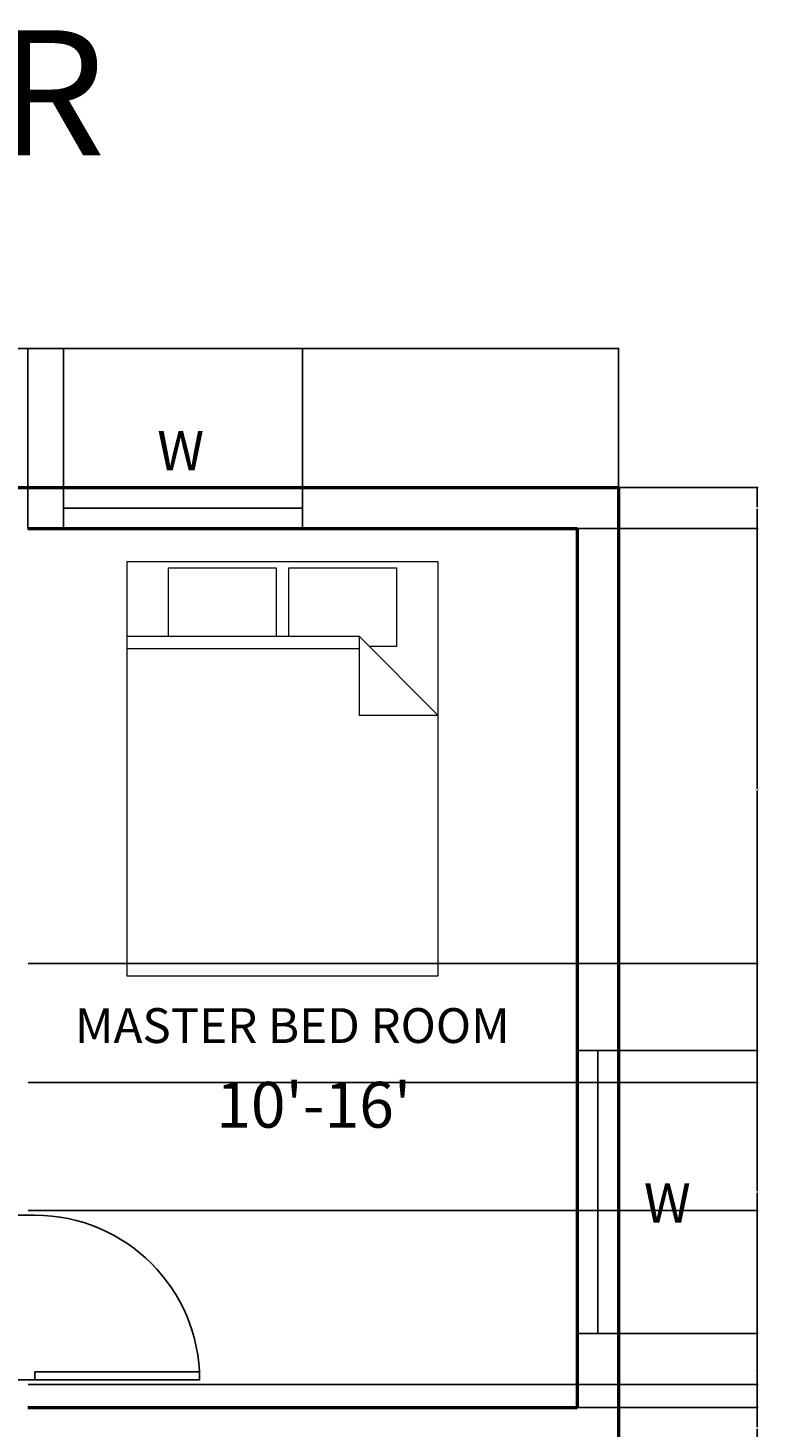
# Model space of a CAD drawing. Units: inches. Extents: x 2164 to 3752, y 2015 to 2629.
# Tile 8 of 8: x 3592 to 3752, y 2323 to 2629. Entities that reach past the tile are written whole.
import ezdxf
from ezdxf.enums import TextEntityAlignment as Align

# ---------------------------------------------------------------- set-up
doc = ezdxf.new("R2010")
doc.units = ezdxf.units.IN
for name, color, linetype, lineweight in [('A-ANNO-DIMS', 2, 'Continuous', 18), ('A-ANNO-TEXT', 7, 'Continuous', 25), ('A-AREA-IDEN', 3, 'Continuous', 25), ('A-DOOR', 3, 'Continuous', 25), ('A-FURN', 8, 'Continuous', 18), ('A-GLAZ', 4, 'Continuous', 25), ('A-WALL', 7, 'Continuous', 50)]:
    doc.layers.add(name, color=color, linetype=linetype, lineweight=lineweight)
doc.styles.get("Standard").update_dxf_attribs({"font": 'arial.ttf'})
doc.dimstyles.get("Standard").update_dxf_attribs({"dimtxt": 0.18, "dimasz": 0.18, "dimexe": 0.18, "dimexo": 0.0625, "dimgap": 0.09, "dimtad": 0, "dimtih": 1, "dimtoh": 1, "dimdec": 4, "dimzin": 0, "dimdsep": 46, "dimtxsty": 'Standard', "dimcen": 0.09, "dimadec": 0, "dimazin": 0, "dimtfac": 1, "dimtdec": 4, "dimtofl": 0, "dimtmove": 0, "dimatfit": 3, "dimfxl": 1, "dimtolj": 1, "dimtzin": 0, "dimarcsym": 0})

# ---------------------------------------------------------------- blocks, each defined once
blk = doc.blocks.new('*U6')
for p, q in [((0, 0), (0, -6)), ((36, 0), (36, -6))]:
    blk.add_line(p, q)
blk.add_lwpolyline([(0, 0), (0, 36), (1.75, 36), (1.75, 0)], close=True)
blk.add_arc((0, 0), 36, 0, 90)
blk = doc.blocks.new('Bed - Queen')
for p, q in [((0, -80.00003), (0, 0)), ((0, 0), (59.99999, 0)), ((59.99999, 0), (59.99999, -80.00003)), ((7.99999, -1.2), (28.79998, -1.2)), ((7.99999, -14.4), (7.99999, -1.2)), ((28.79998, -1.2), (28.79998, -14.4)), ((31.19999, -1.2), (51.99999, -1.2)), ((31.19999, -14.4), (31.19999, -1.2)), ((51.99999, -1.2), (51.99999, -16.4)), ((0, -14.4), (44.8, -14.4)), ((59.99999, -29.6), (44.8, -14.4)), ((44.8, -14.4), (44.8, -29.6)), ((44.8, -16.8), (0, -16.8)), ((51.99999, -16.4), (46.79936, -16.4)), ((44.8, -29.6), (59.99999, -29.6)), ((59.99999, -80.00003), (0, -80.00003))]:
    blk.add_line(p, q)
blk = doc.blocks.new('*D103')
at = {"layer": 'A-ANNO-DIMS', "color": 0, "lineweight": -2, "transparency": 16777216}
for p, q in [((3565.97, 2528.78), (3565.97, 2559.25)), ((3566.15, 2559.07), (3582.66, 2559.07)), ((3599.96, 2559.07), (3583.45, 2559.07)), ((3600.14, 2528.78), (3600.14, 2559.25))]:
    blk.add_line(p, q, dxfattribs=at)
at = {"layer": 'A-ANNO-DIMS', "color": 0, "transparency": 16777216}
for points in [[(3566.15, 2559.1), (3566.15, 2559.04), (3565.97, 2559.07)], [(3599.96, 2559.1), (3599.96, 2559.04), (3600.14, 2559.07)]]:
    blk.add_solid(points, dxfattribs=at)
at = {"layer": 'Defpoints', "color": 0, "transparency": 16777216}
for p in [(3600.14, 2559.07), (3565.97, 2528.72), (3600.14, 2528.72)]:
    blk.add_point(p, dxfattribs=at)
at = {"layer": 'A-ANNO-DIMS', "color": 0, "transparency": 16777216, "insert": (3583.05, 2559.07), "char_height": 0.18, "attachment_point": 5}
blk.add_mtext('\\A1;34.17', dxfattribs=at)
blk = doc.blocks.new('*D104')
at = {"layer": 'A-ANNO-DIMS', "color": 0, "lineweight": -2, "transparency": 16777216}
for p, q in [((3600.14, 2528.78), (3600.14, 2559.25)), ((3600.32, 2559.07), (3625.87, 2559.07)), ((3652.17, 2559.07), (3626.62, 2559.07)), ((3652.35, 2528.78), (3652.35, 2559.25))]:
    blk.add_line(p, q, dxfattribs=at)
at = {"layer": 'A-ANNO-DIMS', "color": 0, "transparency": 16777216}
for points in [[(3600.32, 2559.1), (3600.32, 2559.04), (3600.14, 2559.07)], [(3652.17, 2559.1), (3652.17, 2559.04), (3652.35, 2559.07)]]:
    blk.add_solid(points, dxfattribs=at)
at = {"layer": 'Defpoints', "color": 0, "transparency": 16777216}
for p in [(3652.35, 2559.07), (3600.14, 2528.72), (3652.35, 2528.72)]:
    blk.add_point(p, dxfattribs=at)
at = {"layer": 'A-ANNO-DIMS', "color": 0, "transparency": 16777216, "insert": (3626.25, 2559.07), "char_height": 0.18, "attachment_point": 5}
blk.add_mtext('\\A1;52.21', dxfattribs=at)
blk = doc.blocks.new('*D105')
at = {"layer": 'A-ANNO-DIMS', "color": 0, "lineweight": -2, "transparency": 16777216}
for p, q in [((3652.35, 2528.78), (3652.35, 2559.25)), ((3652.53, 2559.07), (3686.48, 2559.07)), ((3721.21, 2559.07), (3687.27, 2559.07)), ((3721.39, 2528.78), (3721.39, 2559.25))]:
    blk.add_line(p, q, dxfattribs=at)
at = {"layer": 'A-ANNO-DIMS', "color": 0, "transparency": 16777216}
for points in [[(3652.53, 2559.1), (3652.53, 2559.04), (3652.35, 2559.07)], [(3721.21, 2559.1), (3721.21, 2559.04), (3721.39, 2559.07)]]:
    blk.add_solid(points, dxfattribs=at)
at = {"layer": 'Defpoints', "color": 0, "transparency": 16777216}
for p in [(3721.39, 2559.07), (3652.35, 2528.72), (3721.39, 2528.72)]:
    blk.add_point(p, dxfattribs=at)
at = {"layer": 'A-ANNO-DIMS', "color": 0, "transparency": 16777216, "insert": (3686.87, 2559.07), "char_height": 0.18, "attachment_point": 5}
blk.add_mtext('\\A1;69.04', dxfattribs=at)
blk = doc.blocks.new('*D106')
at = {"layer": 'A-ANNO-DIMS', "color": 0, "lineweight": -2, "transparency": 16777216}
for p, q in [((3325.39, 2528.78), (3325.39, 2559.25)), ((3325.57, 2559.07), (3523.11, 2559.07)), ((3721.21, 2559.07), (3523.68, 2559.07)), ((3721.39, 2528.78), (3721.39, 2559.25))]:
    blk.add_line(p, q, dxfattribs=at)
at = {"layer": 'A-ANNO-DIMS', "color": 0, "transparency": 16777216}
for points in [[(3325.57, 2559.1), (3325.57, 2559.04), (3325.39, 2559.07)], [(3721.21, 2559.1), (3721.21, 2559.04), (3721.39, 2559.07)]]:
    blk.add_solid(points, dxfattribs=at)
at = {"layer": 'Defpoints', "color": 0, "transparency": 16777216}
for p in [(3721.39, 2559.07), (3325.39, 2528.72), (3721.39, 2528.72)]:
    blk.add_point(p, dxfattribs=at)
at = {"layer": 'A-ANNO-DIMS', "color": 0, "transparency": 16777216, "insert": (3523.39, 2559.07), "char_height": 0.18, "attachment_point": 5}
blk.add_mtext('\\A1;396', dxfattribs=at)
blk = doc.blocks.new('*D110')
at = {"layer": 'A-ANNO-DIMS', "color": 0, "lineweight": -2, "transparency": 16777216}
for p, q in [((3583.39, 2519.78), (3583.39, 2559.25)), ((3583.57, 2559.07), (3587.75, 2559.07)), ((3592.21, 2559.07), (3588.04, 2559.07)), ((3592.39, 2519.78), (3592.39, 2559.25))]:
    blk.add_line(p, q, dxfattribs=at)
at = {"layer": 'A-ANNO-DIMS', "color": 0, "transparency": 16777216}
for points in [[(3583.57, 2559.1), (3583.57, 2559.04), (3583.39, 2559.07)], [(3592.21, 2559.1), (3592.21, 2559.04), (3592.39, 2559.07)]]:
    blk.add_solid(points, dxfattribs=at)
at = {"layer": 'Defpoints', "color": 0, "transparency": 16777216}
for p in [(3592.39, 2559.07), (3583.39, 2519.72), (3592.39, 2519.72)]:
    blk.add_point(p, dxfattribs=at)
at = {"layer": 'A-ANNO-DIMS', "color": 0, "transparency": 16777216, "insert": (3587.89, 2559.07), "char_height": 0.18, "attachment_point": 5}
blk.add_mtext('\\A1;9', dxfattribs=at)
blk = doc.blocks.new('*D134')
at = {"layer": 'A-ANNO-DIMS', "color": 0, "lineweight": -2, "transparency": 16777216}
for p, q in [((3712.46, 2327.72), (3751.92, 2327.72)), ((3751.74, 2327.54), (3751.74, 2323.4)), ((3751.74, 2318.9), (3751.74, 2323.04)), ((3712.46, 2318.72), (3751.92, 2318.72))]:
    blk.add_line(p, q, dxfattribs=at)
at = {"layer": 'A-ANNO-DIMS', "color": 0, "transparency": 16777216}
for points in [[(3751.71, 2327.54), (3751.77, 2327.54), (3751.74, 2327.72)], [(3751.71, 2318.9), (3751.77, 2318.9), (3751.74, 2318.72)]]:
    blk.add_solid(points, dxfattribs=at)
at = {"layer": 'Defpoints', "color": 0, "transparency": 16777216}
for p in [(3712.39, 2327.72), (3751.74, 2327.72), (3712.39, 2318.72)]:
    blk.add_point(p, dxfattribs=at)
at = {"layer": 'A-ANNO-DIMS', "color": 0, "transparency": 16777216, "insert": (3751.74, 2323.22), "char_height": 0.18, "attachment_point": 5}
blk.add_mtext('\\A1;9', dxfattribs=at)
blk = doc.blocks.new('*D135')
at = {"layer": 'A-ANNO-DIMS', "color": 0, "lineweight": -2, "transparency": 16777216}
for p, q in [((3721.46, 2343.89), (3751.92, 2343.89)), ((3751.74, 2343.71), (3751.74, 2335.98)), ((3751.74, 2327.9), (3751.74, 2335.62)), ((3712.46, 2327.72), (3751.92, 2327.72))]:
    blk.add_line(p, q, dxfattribs=at)
at = {"layer": 'A-ANNO-DIMS', "color": 0, "transparency": 16777216}
for points in [[(3751.71, 2343.71), (3751.77, 2343.71), (3751.74, 2343.89)], [(3751.71, 2327.9), (3751.77, 2327.9), (3751.74, 2327.72)]]:
    blk.add_solid(points, dxfattribs=at)
at = {"layer": 'Defpoints', "color": 0, "transparency": 16777216}
for p in [(3721.39, 2343.89), (3751.74, 2343.89), (3712.39, 2327.72)]:
    blk.add_point(p, dxfattribs=at)
at = {"layer": 'A-ANNO-DIMS', "color": 0, "transparency": 16777216, "insert": (3751.74, 2335.8), "char_height": 0.18, "attachment_point": 5}
blk.add_mtext('\\A1;16.17', dxfattribs=at)
blk = doc.blocks.new('*D136')
at = {"layer": 'A-ANNO-DIMS', "color": 0, "lineweight": -2, "transparency": 16777216}
for p, q in [((3721.46, 2405.68), (3751.92, 2405.68)), ((3751.74, 2405.5), (3751.74, 2374.97)), ((3751.74, 2344.07), (3751.74, 2374.6)), ((3721.46, 2343.89), (3751.92, 2343.89))]:
    blk.add_line(p, q, dxfattribs=at)
at = {"layer": 'A-ANNO-DIMS', "color": 0, "transparency": 16777216}
for points in [[(3751.71, 2405.5), (3751.77, 2405.5), (3751.74, 2405.68)], [(3751.71, 2344.07), (3751.77, 2344.07), (3751.74, 2343.89)]]:
    blk.add_solid(points, dxfattribs=at)
at = {"layer": 'Defpoints', "color": 0, "transparency": 16777216}
for p in [(3721.39, 2405.68), (3751.74, 2405.68), (3721.39, 2343.89)]:
    blk.add_point(p, dxfattribs=at)
at = {"layer": 'A-ANNO-DIMS', "color": 0, "transparency": 16777216, "insert": (3751.74, 2374.78), "char_height": 0.18, "attachment_point": 5}
blk.add_mtext('\\A1;61.8', dxfattribs=at)
blk = doc.blocks.new('*D137')
at = {"layer": 'A-ANNO-DIMS', "color": 0, "lineweight": -2, "transparency": 16777216}
for p, q in [((3712.46, 2519.72), (3751.92, 2519.72)), ((3751.74, 2519.54), (3751.74, 2462.88)), ((3751.74, 2405.86), (3751.74, 2462.52)), ((3721.46, 2405.68), (3751.92, 2405.68))]:
    blk.add_line(p, q, dxfattribs=at)
at = {"layer": 'A-ANNO-DIMS', "color": 0, "transparency": 16777216}
for points in [[(3751.71, 2519.54), (3751.77, 2519.54), (3751.74, 2519.72)], [(3751.71, 2405.86), (3751.77, 2405.86), (3751.74, 2405.68)]]:
    blk.add_solid(points, dxfattribs=at)
at = {"layer": 'Defpoints', "color": 0, "transparency": 16777216}
for p in [(3712.39, 2519.72), (3751.74, 2519.72), (3721.39, 2405.68)]:
    blk.add_point(p, dxfattribs=at)
at = {"layer": 'A-ANNO-DIMS', "color": 0, "transparency": 16777216, "insert": (3751.74, 2462.7), "char_height": 0.18, "attachment_point": 5}
blk.add_mtext('\\A1;114.04', dxfattribs=at)
blk = doc.blocks.new('*D138')
at = {"layer": 'A-ANNO-DIMS', "color": 0, "lineweight": -2, "transparency": 16777216}
for p, q in [((3721.46, 2528.72), (3751.92, 2528.72)), ((3751.74, 2528.54), (3751.74, 2524.4)), ((3751.74, 2519.9), (3751.74, 2524.04)), ((3712.46, 2519.72), (3751.92, 2519.72))]:
    blk.add_line(p, q, dxfattribs=at)
at = {"layer": 'A-ANNO-DIMS', "color": 0, "transparency": 16777216}
for points in [[(3751.71, 2528.54), (3751.77, 2528.54), (3751.74, 2528.72)], [(3751.71, 2519.9), (3751.77, 2519.9), (3751.74, 2519.72)]]:
    blk.add_solid(points, dxfattribs=at)
at = {"layer": 'Defpoints', "color": 0, "transparency": 16777216}
for p in [(3721.39, 2528.72), (3751.74, 2528.72), (3712.39, 2519.72)]:
    blk.add_point(p, dxfattribs=at)
at = {"layer": 'A-ANNO-DIMS', "color": 0, "transparency": 16777216, "insert": (3751.74, 2524.22), "char_height": 0.18, "attachment_point": 5}
blk.add_mtext('\\A1;9', dxfattribs=at)
blk = doc.blocks.new('*D145')
at = {"layer": 'A-ANNO-DIMS', "color": 0, "lineweight": -2, "transparency": 16777216}
for p, q in [((3592.46, 2424.72), (3751.92, 2424.72)), ((3751.74, 2424.54), (3751.74, 2411.9)), ((3751.74, 2398.9), (3751.74, 2411.54)), ((3592.46, 2398.72), (3751.92, 2398.72))]:
    blk.add_line(p, q, dxfattribs=at)
at = {"layer": 'A-ANNO-DIMS', "color": 0, "transparency": 16777216}
for points in [[(3751.71, 2424.54), (3751.77, 2424.54), (3751.74, 2424.72)], [(3751.71, 2398.9), (3751.77, 2398.9), (3751.74, 2398.72)]]:
    blk.add_solid(points, dxfattribs=at)
at = {"layer": 'Defpoints', "color": 0, "transparency": 16777216}
for p in [(3592.39, 2424.72), (3751.74, 2424.72), (3592.39, 2398.72)]:
    blk.add_point(p, dxfattribs=at)
at = {"layer": 'A-ANNO-DIMS', "color": 0, "transparency": 16777216, "insert": (3751.74, 2411.72), "char_height": 0.18, "attachment_point": 5}
blk.add_mtext('\\A1;26', dxfattribs=at)
blk = doc.blocks.new('*D147')
at = {"layer": 'A-ANNO-DIMS', "color": 0, "lineweight": -2, "transparency": 16777216}
for p, q in [((3592.46, 2370.72), (3751.92, 2370.72)), ((3751.74, 2370.54), (3751.74, 2351.9)), ((3751.74, 2332.9), (3751.74, 2351.54)), ((3592.46, 2332.72), (3751.92, 2332.72))]:
    blk.add_line(p, q, dxfattribs=at)
at = {"layer": 'A-ANNO-DIMS', "color": 0, "transparency": 16777216}
for points in [[(3751.71, 2370.54), (3751.77, 2370.54), (3751.74, 2370.72)], [(3751.71, 2332.9), (3751.77, 2332.9), (3751.74, 2332.72)]]:
    blk.add_solid(points, dxfattribs=at)
at = {"layer": 'Defpoints', "color": 0, "transparency": 16777216}
for p in [(3592.39, 2370.72), (3751.74, 2370.72), (3592.39, 2332.72)]:
    blk.add_point(p, dxfattribs=at)
at = {"layer": 'A-ANNO-DIMS', "color": 0, "transparency": 16777216, "insert": (3751.74, 2351.72), "char_height": 0.18, "attachment_point": 5}
blk.add_mtext('\\A1;38', dxfattribs=at)

msp = doc.modelspace()

# ---------------------------------------------------------------- linework, layer by layer
at = {"layer": 'A-GLAZ'}
for p, q in [((3600.1393, 2528.7172), (3600.1393, 2519.7172)), ((3652.3529, 2528.7172), (3652.395, 2519.7172)), ((3652.374, 2524.2172), (3600.1393, 2524.2172)), ((3712.395, 2405.6818), (3721.395, 2405.6818)), ((3716.895, 2405.6818), (3716.895, 2343.8868)), ((3712.395, 2343.8868), (3721.395, 2343.8868))]:
    msp.add_line(p, q, dxfattribs=at)
at = {"layer": 'A-WALL'}
for p, q in [((3325.395, 2528.7172), (3721.395, 2528.7172)), ((3721.395, 2528.7172), (3721.395, 2045.7172)), ((3592.395, 2519.7172), (3712.395, 2519.7172)), ((3712.395, 2519.7172), (3712.395, 2327.7172)), ((3592.395, 2327.7172), (3712.395, 2327.7172))]:
    msp.add_line(p, q, dxfattribs=at)

# ---------------------------------------------------------------- block references
at = {"layer": 'A-DOOR', "xscale": -1, "rotation": 270}
msp.add_blockref('*U6', (3593.895, 2333.7172), dxfattribs=at)
at = {"layer": 'A-FURN', "xscale": 1.1322848164304, "yscale": 1.1322848164304, "zscale": 1.1322848164304}
msp.add_blockref('Bed - Queen', (3614.0367, 2512.4991), dxfattribs=at)

# ---------------------------------------------------------------- texts
at = {"layer": 'A-ANNO-TEXT'}
for s, height, p in [('FIRST FLOOR', 27.32215, (3495.4066, 2611.4091)), ('W', 8.5558, (3625.7582, 2535.6454)), ('W', 8.5558, (3732.0801, 2371.2829))]:
    msp.add_text(s, height=height, dxfattribs=at).set_placement(p, align=Align.MIDDLE)
at = {"layer": 'A-AREA-IDEN'}
for s, height, p in [('MASTER BED ROOM', 7.606933, (3602.6596, 2407.337)), ("10'-16'", 10, (3633.5277, 2388.8358))]:
    msp.add_text(s, height=height, dxfattribs=at).set_placement(p)

# ---------------------------------------------------------------- dimensions: what is measured, and where the dimension line sits
at = {"layer": 'A-ANNO-DIMS'}
for base, p1, p2, override, picture, middle in [((3721.395, 2559.0672), (3325.395, 2528.7172), (3721.395, 2528.7172), {"dimdec": 0, "dimlfac": 1, "dimrnd": 0, "dimzin": 0, "dimdsep": 46, "dimlunit": 2}, '*D106', (3523.395, 2559.0672)), ((3600.1393, 2559.0672), (3565.9689, 2528.7172), (3600.1393, 2528.7172), {"dimdec": 2, "dimlfac": 1, "dimrnd": 0, "dimzin": 0, "dimdsep": 46, "dimlunit": 2}, '*D103', (3583.0541, 2559.0672)), ((3592.395, 2559.0672), (3583.395, 2519.7172), (3592.395, 2519.7172), {"dimdec": 0, "dimlfac": 1, "dimrnd": 0, "dimzin": 0, "dimdsep": 46, "dimlunit": 2}, '*D110', (3587.895, 2559.0672)), ((3652.3529, 2559.0672), (3600.1393, 2528.7172), (3652.3529, 2528.7172), {"dimdec": 2, "dimlfac": 1, "dimrnd": 0, "dimzin": 0, "dimdsep": 46, "dimlunit": 2}, '*D104', (3626.2461, 2559.0672)), ((3721.395, 2559.0672), (3652.3529, 2528.7172), (3721.395, 2528.7172), {"dimdec": 2, "dimlfac": 1, "dimrnd": 0, "dimzin": 0, "dimdsep": 46, "dimlunit": 2}, '*D105', (3686.874, 2559.0672))]:
    dim = msp.add_linear_dim(base=base, p1=p1, p2=p2, dimstyle='Standard', override=override, dxfattribs=at)
    dim.commit()
    dim.dimension.update_dxf_attribs({"geometry": picture, "text_midpoint": middle})
for base, p1, p2, override, picture, middle in [((3751.745, 2528.7172), (3712.395, 2519.7172), (3721.395, 2528.7172), {"dimdec": 0, "dimlfac": 1, "dimrnd": 0, "dimzin": 0, "dimdsep": 46, "dimlunit": 2}, '*D138', (3751.745, 2524.2172)), ((3751.745, 2519.7172), (3721.395, 2405.6818), (3712.395, 2519.7172), {"dimdec": 2, "dimlfac": 1, "dimrnd": 0, "dimzin": 0, "dimdsep": 46, "dimlunit": 2}, '*D137', (3751.745, 2462.6995)), ((3751.745, 2424.7172), (3592.395, 2398.7172), (3592.395, 2424.7172), {"dimdec": 0, "dimlfac": 1, "dimrnd": 0, "dimzin": 0, "dimdsep": 46, "dimlunit": 2}, '*D145', (3751.745, 2411.7172)), ((3751.745, 2405.6818), (3721.395, 2343.8868), (3721.395, 2405.6818), {"dimdec": 1, "dimlfac": 1, "dimrnd": 0, "dimzin": 0, "dimdsep": 46, "dimlunit": 2}, '*D136', (3751.745, 2374.7843)), ((3751.745, 2370.7172), (3592.395, 2332.7172), (3592.395, 2370.7172), {"dimdec": 0, "dimlfac": 1, "dimrnd": 0, "dimzin": 0, "dimdsep": 46, "dimlunit": 2}, '*D147', (3751.745, 2351.7172)), ((3751.745, 2343.8868), (3712.395, 2327.7172), (3721.395, 2343.8868), {"dimdec": 2, "dimlfac": 1, "dimrnd": 0, "dimzin": 0, "dimdsep": 46, "dimlunit": 2}, '*D135', (3751.745, 2335.802)), ((3751.745, 2327.7172), (3712.395, 2318.7172), (3712.395, 2327.7172), {"dimdec": 0, "dimlfac": 1, "dimrnd": 0, "dimzin": 0, "dimdsep": 46, "dimlunit": 2}, '*D134', (3751.745, 2323.2172))]:
    dim = msp.add_linear_dim(base=base, p1=p1, p2=p2, angle=90, dimstyle='Standard', override=override, dxfattribs=at)
    dim.commit()
    dim.dimension.update_dxf_attribs({"geometry": picture, "text_midpoint": middle})

doc.saveas('drawing.dxf')
